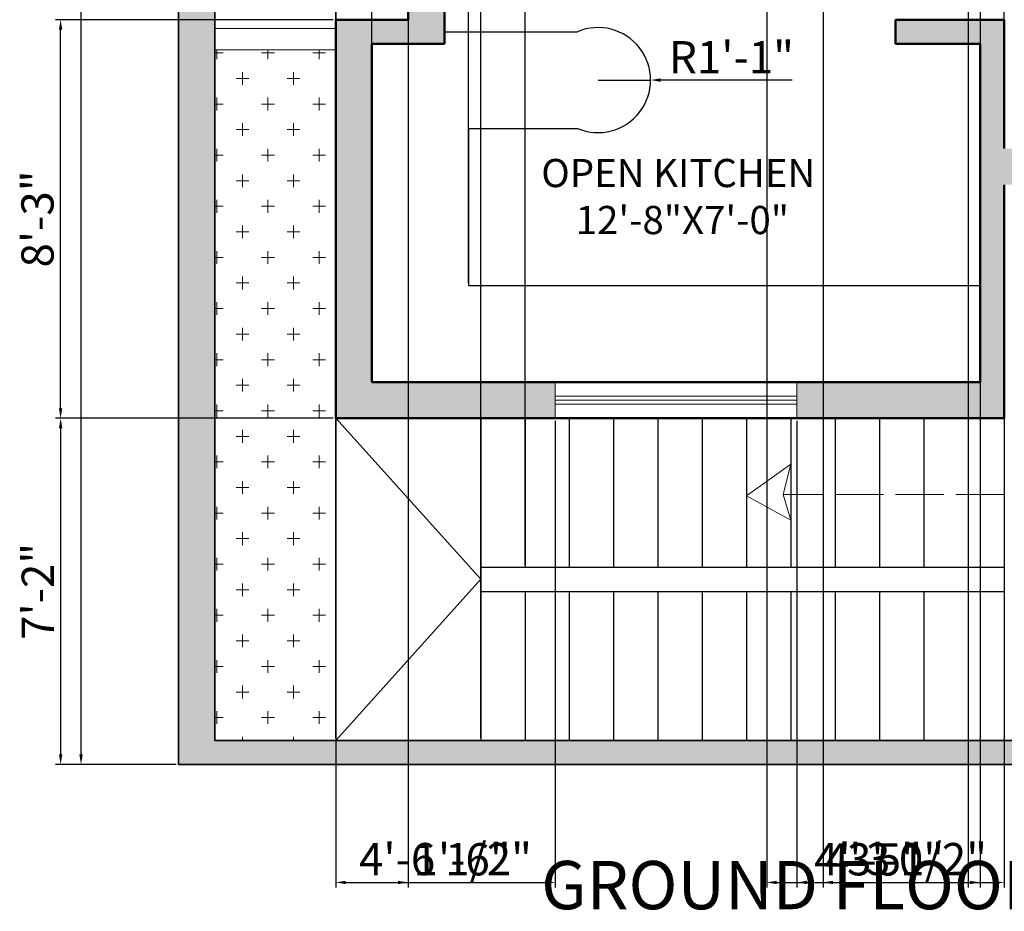
# Model space of a CAD drawing. Units: inches. Extents: x 1369 to 1844, y 2136 to 2743.
# Tile 1 of 4: x 1375 to 1620, y 2136 to 2358. Entities that reach past the tile are written whole.
import ezdxf

# ---------------------------------------------------------------- set-up
doc = ezdxf.new("R2010")
doc.units = ezdxf.units.IN
doc.linetypes.add('ACAD_ISO02W100', pattern=[15, 12, -3])
for name, color, linetype, lineweight in [('A-ANNO-DIMS', 2, 'Continuous', 18), ('A-ANNO-SYMB', 7, 'Continuous', 18), ('A-ANNO-TEXT', 7, 'Continuous', 25), ('A-AREA-IDEN', 7, 'Continuous', 25), ('A-FLOR-CASE', 8, 'Continuous', 25), ('A-FLOR-PATT', 9, 'Continuous', 13), ('A-FLOR-STRS', 7, 'Continuous', 25), ('A-FLOR-STRS-PATH', 7, 'ACAD_ISO02W100', 18), ('A-WALL', 7, 'Continuous', 50), ('C-PROP', 7, 'Continuous', 35), ('L-PLNT', 3, 'Continuous', 18)]:
    doc.layers.add(name, color=color, linetype=linetype, lineweight=lineweight)
for name, color, linetype, lineweight, true_color in [('A-GLAZ', 244, 'Continuous', 20, 0x991b1e), ('A-WALL-PATT', 251, 'Continuous', 13, 0x636466), ('C-PROP-PATT', 251, 'Continuous', 13, 0x636466), ('L-PLNT-PATT', 116, 'Continuous', 13, 0x136734)]:
    doc.layers.add(name, color=color, linetype=linetype, lineweight=lineweight, true_color=true_color)
doc.styles.get("Standard").update_dxf_attribs({"font": 'arial.ttf'})
doc.dimstyles.new('ISO-25', dxfattribs={"dimtxt": 8, "dimasz": 2.5, "dimexe": 1.25, "dimexo": 0.625, "dimtad": 1, "dimlunit": 3, "dimtxsty": 'Standard', "dimcen": 2.5, "dimadec": 0, "dimazin": 0, "dimtfac": 1, "dimtmove": 0, "dimatfit": 3, "dimfxl": 1, "dimarcsym": 0})

# ---------------------------------------------------------------- blocks, each defined once
blk = doc.blocks.new('*D12')
at = {"layer": 'A-ANNO-DIMS', "color": 0, "lineweight": -2, "transparency": 16777216}
for p, q in [((1413.89, 2682.76), (1389.03, 2682.76)), ((1390.28, 2175.26), (1390.28, 2680.26)), ((1413.89, 2172.76), (1389.03, 2172.76))]:
    blk.add_line(p, q, dxfattribs=at)
at = {"layer": 'A-ANNO-DIMS', "color": 0, "transparency": 16777216}
for points in [[(1389.86, 2680.26), (1390.69, 2680.26), (1390.28, 2682.76)], [(1389.86, 2175.26), (1390.69, 2175.26), (1390.28, 2172.76)]]:
    blk.add_solid(points, dxfattribs=at)
at = {"layer": 'Defpoints', "color": 0, "transparency": 16777216}
for p in [(1390.28, 2682.76), (1414.51, 2682.76), (1414.51, 2172.76)]:
    blk.add_point(p, dxfattribs=at)
at = {"layer": 'A-ANNO-DIMS', "color": 0, "transparency": 16777216, "insert": (1385.57, 2427.76), "char_height": 8, "attachment_point": 5, "rotation": 90}
blk.add_mtext('42\'-6"', dxfattribs=at)
blk = doc.blocks.new('WIN-60IN')
for p, q in [((3.5, 0), (3.5, 60)), ((4.5, 0), (4.5, 60)), ((5.5, 0), (5.5, 60))]:
    blk.add_line(p, q)
blk.add_lwpolyline([(0, 60), (9, 60), (9, 0), (0, 0)], close=True)
blk = doc.blocks.new('*D36')
at = {"layer": 'A-ANNO-DIMS', "color": 0, "lineweight": -2, "transparency": 16777216}
for p, q in [((1452.89, 2258.76), (1383.96, 2258.76)), ((1385.21, 2256.26), (1385.21, 2175.26)), ((1413.89, 2172.76), (1383.96, 2172.76))]:
    blk.add_line(p, q, dxfattribs=at)
at = {"layer": 'A-ANNO-DIMS', "color": 0, "transparency": 16777216}
for points in [[(1384.79, 2256.26), (1385.63, 2256.26), (1385.21, 2258.76)], [(1384.79, 2175.26), (1385.63, 2175.26), (1385.21, 2172.76)]]:
    blk.add_solid(points, dxfattribs=at)
at = {"layer": 'Defpoints', "color": 0, "transparency": 16777216}
for p in [(1453.51, 2258.76), (1385.21, 2172.76), (1414.51, 2172.76)]:
    blk.add_point(p, dxfattribs=at)
at = {"layer": 'A-ANNO-DIMS', "color": 0, "transparency": 16777216, "insert": (1380.57, 2215.76), "char_height": 8, "attachment_point": 5, "rotation": 90}
blk.add_mtext('7\'-2"', dxfattribs=at)
blk = doc.blocks.new('*D37')
at = {"layer": 'A-ANNO-DIMS', "color": 0, "lineweight": -2, "transparency": 16777216}
for p, q in [((1452.89, 2357.76), (1383.96, 2357.76)), ((1385.21, 2261.26), (1385.21, 2355.26)), ((1452.89, 2258.76), (1383.96, 2258.76))]:
    blk.add_line(p, q, dxfattribs=at)
at = {"layer": 'A-ANNO-DIMS', "color": 0, "transparency": 16777216}
for points in [[(1384.79, 2355.26), (1385.63, 2355.26), (1385.21, 2357.76)], [(1384.79, 2261.26), (1385.63, 2261.26), (1385.21, 2258.76)]]:
    blk.add_solid(points, dxfattribs=at)
at = {"layer": 'Defpoints', "color": 0, "transparency": 16777216}
for p in [(1385.21, 2357.76), (1453.51, 2357.76), (1453.51, 2258.76)]:
    blk.add_point(p, dxfattribs=at)
at = {"layer": 'A-ANNO-DIMS', "color": 0, "transparency": 16777216, "insert": (1380.5, 2308.26), "char_height": 8, "attachment_point": 5, "rotation": 90}
blk.add_mtext('8\'-3"', dxfattribs=at)
blk = doc.blocks.new('*D42')
at = {"layer": 'A-ANNO-DIMS', "color": 0, "lineweight": -2, "transparency": 16777216}
for p, q in [((1453.51, 2453.13), (1453.51, 2142.21)), ((1471.51, 2453.13), (1471.51, 2142.21)), ((1456.01, 2143.46), (1469.01, 2143.46)), ((1471.51, 2143.46), (1495.77, 2143.46))]:
    blk.add_line(p, q, dxfattribs=at)
at = {"layer": 'A-ANNO-DIMS', "color": 0, "transparency": 16777216}
for points in [[(1456.01, 2143.87), (1456.01, 2143.04), (1453.51, 2143.46)], [(1469.01, 2143.87), (1469.01, 2143.04), (1471.51, 2143.46)]]:
    blk.add_solid(points, dxfattribs=at)
at = {"layer": 'Defpoints', "color": 0, "transparency": 16777216}
for p in [(1453.51, 2453.76), (1471.51, 2453.76), (1471.51, 2143.46)]:
    blk.add_point(p, dxfattribs=at)
at = {"layer": 'A-ANNO-DIMS', "color": 0, "transparency": 16777216, "insert": (1484.89, 2148.17), "char_height": 8, "attachment_point": 5}
blk.add_mtext('1\'-6"', dxfattribs=at)
blk = doc.blocks.new('*D43')
at = {"layer": 'A-ANNO-DIMS', "color": 0, "lineweight": -2, "transparency": 16777216}
for p, q in [((1453.51, 2258.13), (1453.51, 2142.21)), ((1508.01, 2258.13), (1508.01, 2142.21)), ((1456.01, 2143.46), (1505.51, 2143.46))]:
    blk.add_line(p, q, dxfattribs=at)
at = {"layer": 'A-ANNO-DIMS', "color": 0, "transparency": 16777216}
for points in [[(1456.01, 2143.87), (1456.01, 2143.04), (1453.51, 2143.46)], [(1505.51, 2143.87), (1505.51, 2143.04), (1508.01, 2143.46)]]:
    blk.add_solid(points, dxfattribs=at)
at = {"layer": 'Defpoints', "color": 0, "transparency": 16777216}
for p in [(1453.51, 2258.76), (1508.01, 2258.76), (1508.01, 2143.46)]:
    blk.add_point(p, dxfattribs=at)
at = {"layer": 'A-ANNO-DIMS', "color": 0, "transparency": 16777216, "insert": (1480.76, 2148.22), "char_height": 8, "attachment_point": 5}
blk.add_mtext('4\'-6 1/2"', dxfattribs=at)
blk = doc.blocks.new('*D44')
at = {"layer": 'A-ANNO-DIMS', "color": 0, "lineweight": -2, "transparency": 16777216}
for p, q in [((1568.01, 2258.13), (1568.01, 2142.21)), ((1619.51, 2258.13), (1619.51, 2142.21)), ((1570.51, 2143.46), (1617.01, 2143.46))]:
    blk.add_line(p, q, dxfattribs=at)
at = {"layer": 'A-ANNO-DIMS', "color": 0, "transparency": 16777216}
for points in [[(1570.51, 2143.87), (1570.51, 2143.04), (1568.01, 2143.46)], [(1617.01, 2143.87), (1617.01, 2143.04), (1619.51, 2143.46)]]:
    blk.add_solid(points, dxfattribs=at)
at = {"layer": 'Defpoints', "color": 0, "transparency": 16777216}
for p in [(1568.01, 2258.76), (1619.51, 2258.76), (1619.51, 2143.46)]:
    blk.add_point(p, dxfattribs=at)
at = {"layer": 'A-ANNO-DIMS', "color": 0, "transparency": 16777216, "insert": (1593.76, 2148.22), "char_height": 8, "attachment_point": 5}
blk.add_mtext('4\'-3 1/2"', dxfattribs=at)
blk = doc.blocks.new('*D45')
at = {"layer": 'A-ANNO-DIMS', "color": 0, "lineweight": -2, "transparency": 16777216}
for p, q in [((1619.51, 2326.38), (1619.51, 2734.31)), ((1636.5, 2326.38), (1636.5, 2734.31)), ((1622.01, 2733.06), (1634, 2733.06)), ((1636.5, 2733.06), (1660.77, 2733.06))]:
    blk.add_line(p, q, dxfattribs=at)
at = {"layer": 'A-ANNO-DIMS', "color": 0, "transparency": 16777216}
for points in [[(1622.01, 2733.47), (1622.01, 2732.64), (1619.51, 2733.06)], [(1634, 2733.47), (1634, 2732.64), (1636.5, 2733.06)]]:
    blk.add_solid(points, dxfattribs=at)
at = {"layer": 'Defpoints', "color": 0, "transparency": 16777216}
for p in [(1636.5, 2733.06), (1619.51, 2325.76), (1636.5, 2325.76)]:
    blk.add_point(p, dxfattribs=at)
at = {"layer": 'A-ANNO-DIMS', "color": 0, "transparency": 16777216, "insert": (1649.88, 2737.77), "char_height": 8, "attachment_point": 5}
blk.add_mtext('1\'-5"', dxfattribs=at)
blk = doc.blocks.new('*D49')
at = {"layer": 'A-ANNO-DIMS', "color": 0, "lineweight": -2, "transparency": 16777216}
for p, q in [((1574.51, 2507.13), (1574.51, 2142.21)), ((1610.51, 2507.13), (1610.51, 2142.21)), ((1577.01, 2143.46), (1608.01, 2143.46))]:
    blk.add_line(p, q, dxfattribs=at)
at = {"layer": 'A-ANNO-DIMS', "color": 0, "transparency": 16777216}
for points in [[(1577.01, 2143.87), (1577.01, 2143.04), (1574.51, 2143.46)], [(1608.01, 2143.87), (1608.01, 2143.04), (1610.51, 2143.46)]]:
    blk.add_solid(points, dxfattribs=at)
at = {"layer": 'Defpoints', "color": 0, "transparency": 16777216}
for p in [(1574.51, 2507.76), (1610.51, 2507.76), (1610.51, 2143.46)]:
    blk.add_point(p, dxfattribs=at)
at = {"layer": 'A-ANNO-DIMS', "color": 0, "transparency": 16777216, "insert": (1592.51, 2148.17), "char_height": 8, "attachment_point": 5}
blk.add_mtext('3\'-0"', dxfattribs=at)
blk = doc.blocks.new('*D53')
at = {"layer": 'A-ANNO-DIMS', "color": 0, "lineweight": -2, "transparency": 16777216}
for p, q in [((1613.51, 2469.13), (1613.51, 2142.21)), ((1560.51, 2453.13), (1560.51, 2142.21)), ((1563.01, 2143.46), (1611.01, 2143.46))]:
    blk.add_line(p, q, dxfattribs=at)
at = {"layer": 'A-ANNO-DIMS', "color": 0, "transparency": 16777216}
for points in [[(1563.01, 2143.87), (1563.01, 2143.04), (1560.51, 2143.46)], [(1611.01, 2143.87), (1611.01, 2143.04), (1613.51, 2143.46)]]:
    blk.add_solid(points, dxfattribs=at)
at = {"layer": 'Defpoints', "color": 0, "transparency": 16777216}
for p in [(1613.51, 2469.76), (1560.51, 2453.76), (1613.51, 2143.46)]:
    blk.add_point(p, dxfattribs=at)
at = {"layer": 'A-ANNO-DIMS', "color": 0, "transparency": 16777216, "insert": (1587.01, 2148.15), "char_height": 8, "attachment_point": 5}
blk.add_mtext('4\'-5"', dxfattribs=at)
blk = doc.blocks.new('*D54')
at = {"layer": 'A-ANNO-DIMS', "color": 0, "lineweight": -2, "transparency": 16777216}
for p, q in [((1462.51, 2268.38), (1462.51, 2734.31)), ((1486.51, 2292.38), (1486.51, 2734.31)), ((1465.01, 2733.06), (1484.01, 2733.06))]:
    blk.add_line(p, q, dxfattribs=at)
at = {"layer": 'A-ANNO-DIMS', "color": 0, "transparency": 16777216}
for points in [[(1465.01, 2733.47), (1465.01, 2732.64), (1462.51, 2733.06)], [(1484.01, 2733.47), (1484.01, 2732.64), (1486.51, 2733.06)]]:
    blk.add_solid(points, dxfattribs=at)
at = {"layer": 'Defpoints', "color": 0, "transparency": 16777216}
for p in [(1486.51, 2733.06), (1486.51, 2291.76), (1462.51, 2267.76)]:
    blk.add_point(p, dxfattribs=at)
at = {"layer": 'A-ANNO-DIMS', "color": 0, "transparency": 16777216, "insert": (1474.51, 2737.77), "char_height": 8, "attachment_point": 5}
blk.add_mtext('2\'-0"', dxfattribs=at)
blk = doc.blocks.new('*D55')
at = {"layer": 'A-ANNO-DIMS', "color": 0, "lineweight": -2, "transparency": 16777216}
for p, q in [((1453.51, 2179.38), (1453.51, 2734.31)), ((1489.51, 2179.38), (1489.51, 2734.31)), ((1456.01, 2733.06), (1487.01, 2733.06))]:
    blk.add_line(p, q, dxfattribs=at)
at = {"layer": 'A-ANNO-DIMS', "color": 0, "transparency": 16777216}
for points in [[(1456.01, 2733.47), (1456.01, 2732.64), (1453.51, 2733.06)], [(1487.01, 2733.47), (1487.01, 2732.64), (1489.51, 2733.06)]]:
    blk.add_solid(points, dxfattribs=at)
at = {"layer": 'Defpoints', "color": 0, "transparency": 16777216}
for p in [(1489.51, 2733.06), (1453.51, 2178.76), (1489.51, 2178.76)]:
    blk.add_point(p, dxfattribs=at)
at = {"layer": 'A-ANNO-DIMS', "color": 0, "transparency": 16777216, "insert": (1471.51, 2737.77), "char_height": 8, "attachment_point": 5}
blk.add_mtext('3\'-0"', dxfattribs=at)
blk = doc.blocks.new('*D56')
at = {"layer": 'A-ANNO-DIMS', "color": 0, "lineweight": -2, "transparency": 16777216}
for p, q in [((1489.51, 2222.38), (1489.51, 2734.31)), ((1500.51, 2222.38), (1500.51, 2734.31)), ((1492.01, 2733.06), (1498.01, 2733.06)), ((1500.51, 2733.06), (1531.74, 2733.06))]:
    blk.add_line(p, q, dxfattribs=at)
at = {"layer": 'A-ANNO-DIMS', "color": 0, "transparency": 16777216}
for points in [[(1492.01, 2733.47), (1492.01, 2732.64), (1489.51, 2733.06)], [(1498.01, 2733.47), (1498.01, 2732.64), (1500.51, 2733.06)]]:
    blk.add_solid(points, dxfattribs=at)
at = {"layer": 'Defpoints', "color": 0, "transparency": 16777216}
for p in [(1500.51, 2733.06), (1489.51, 2221.76), (1500.51, 2221.76)]:
    blk.add_point(p, dxfattribs=at)
at = {"layer": 'A-ANNO-DIMS', "color": 0, "transparency": 16777216, "insert": (1517.38, 2737.77), "char_height": 8, "attachment_point": 5}
blk.add_mtext('0\'-11"', dxfattribs=at)
blk = doc.blocks.new('*D57')
at = {"layer": 'A-ANNO-DIMS', "color": 0, "lineweight": -2, "transparency": 16777216}
for p, q in [((1518.64, 2342.76), (1531.68, 2342.76)), ((1566.86, 2342.76), (1534.18, 2342.76))]:
    blk.add_line(p, q, dxfattribs=at)
at = {"layer": 'A-ANNO-DIMS', "color": 0, "transparency": 16777216}
blk.add_solid([(1534.18, 2343.17), (1534.18, 2342.34), (1531.68, 2342.76)], dxfattribs=at)
at = {"layer": 'Defpoints', "color": 0, "transparency": 16777216}
for p in [(1518.64, 2342.76), (1531.68, 2342.76)]:
    blk.add_point(p, dxfattribs=at)
at = {"layer": 'A-ANNO-DIMS', "color": 0, "transparency": 16777216, "insert": (1551.77, 2347.4), "char_height": 8, "attachment_point": 5, "rotation": 359.9999}
blk.add_mtext('R1\'-1"', dxfattribs=at)

msp = doc.modelspace()

# ---------------------------------------------------------------- hatches: boundary and pattern name
at = {"layer": 'A-WALL-PATT'}
h = msp.add_hatch(color=256, dxfattribs=at)
h.dxf.hatch_style = 1
h.paths.add_polyline_path([(1619.511, 2460.756), (1768.511, 2460.756), (1768.511, 2444.065), (1777.511, 2444.065), (1777.511, 2498.256), (1768.511, 2498.256), (1768.511, 2466.756), (1619.511, 2466.756), (1619.511, 2469.756), (1614.511, 2469.756), (1613.511, 2469.756), (1613.511, 2433.756), (1619.511, 2433.756)])
h.paths.add_polyline_path([(1480.511, 2453.756), (1560.511, 2453.756), (1560.511, 2474.756), (1556.011, 2474.756), (1554.511, 2474.756), (1554.511, 2459.756), (1462.511, 2459.756), (1462.511, 2473.256), (1453.511, 2473.256), (1453.511, 2453.756), (1471.511, 2453.756), (1471.511, 2390.756), (1480.511, 2390.756)])
h.paths.add_polyline_path([(1574.511, 2513.156), (1574.511, 2513.756), (1462.511, 2513.756), (1462.511, 2551.882), (1453.511, 2551.882), (1453.511, 2494.256), (1462.511, 2494.256), (1462.511, 2507.756), (1554.511, 2507.756), (1554.511, 2504.756), (1556.011, 2504.756), (1560.511, 2504.756), (1560.511, 2507.756), (1574.511, 2507.756)])
h.paths.add_polyline_path([(1462.511, 2351.756), (1480.511, 2351.756), (1480.511, 2357.756), (1480.511, 2360.756), (1476.011, 2360.756), (1471.511, 2360.756), (1471.511, 2357.756), (1453.511, 2357.756), (1453.511, 2258.756), (1508.011, 2258.756), (1508.011, 2267.756), (1462.511, 2267.756)])
h.paths.add_polyline_path([(1619.511, 2357.756), (1592.511, 2357.756), (1592.511, 2351.756), (1613.511, 2351.756), (1613.511, 2267.756), (1568.011, 2267.756), (1568.011, 2258.756), (1619.511, 2258.756), (1619.511, 2316.756), (1636.503, 2316.756), (1636.503, 2325.756), (1619.511, 2325.756)])
h.paths.add_polyline_path([(1717.511, 2323.956), (1717.511, 2325.756), (1696.503, 2325.756), (1696.503, 2316.756), (1717.511, 2316.756)])
h.paths.add_polyline_path([(1777.511, 2384.065), (1768.511, 2384.065), (1768.511, 2325.756), (1765.511, 2325.756), (1765.511, 2323.956), (1765.511, 2316.756), (1777.511, 2316.756)])
h.paths.add_polyline_path([(1777.511, 2652.756), (1731.511, 2652.756), (1731.511, 2643.756), (1768.511, 2643.756), (1768.511, 2595.756), (1673.511, 2595.756), (1673.511, 2598.756), (1672.011, 2598.756), (1667.511, 2598.756), (1667.511, 2595.756), (1613.511, 2595.756), (1613.511, 2513.756), (1610.511, 2513.756), (1610.511, 2513.156), (1610.511, 2507.756), (1613.511, 2507.756), (1613.511, 2505.756), (1619.511, 2505.756), (1619.511, 2589.756), (1768.511, 2589.756), (1768.511, 2558.256), (1777.511, 2558.256)])
h.paths.add_polyline_path([(1710.511, 2652.756), (1616.643, 2652.756), (1616.643, 2643.756), (1667.511, 2643.756), (1667.511, 2628.756), (1672.011, 2628.756), (1673.511, 2628.756), (1673.511, 2643.756), (1710.511, 2643.756)], flags=17)
h.paths.add_polyline_path([(1556.643, 2652.756), (1453.511, 2652.756), (1453.511, 2611.882), (1462.511, 2611.882), (1462.511, 2643.756), (1556.643, 2643.756)])
at = {"layer": 'C-PROP-PATT'}
h = msp.add_hatch(color=256, dxfattribs=at)
h.dxf.hatch_style = 1
h.paths.add_polyline_path([(1423.511, 2676.756), (1801.511, 2676.756), (1801.511, 2178.756), (1777.511, 2178.756), (1777.511, 2172.756), (1807.511, 2172.756), (1807.511, 2682.756), (1414.511, 2682.756), (1414.511, 2172.756), (1642.884, 2172.756), (1642.884, 2178.756), (1423.511, 2178.756)])
at = {"layer": 'L-PLNT-PATT'}
h = msp.add_hatch(dxfattribs=at)
h.set_pattern_fill('CROSS', color=256)
h.paths.add_polyline_path([(1453.511, 2652.756), (1777.511, 2652.756), (1788.511, 2652.756), (1788.511, 2178.756), (1801.511, 2178.756), (1801.511, 2676.756), (1423.511, 2676.756), (1423.511, 2453.756), (1453.511, 2453.756)])
h.paths.add_polyline_path([(1453.511, 2350.279), (1423.511, 2350.279), (1423.511, 2178.756), (1453.511, 2178.756), (1453.511, 2258.756)], flags=17)

# ---------------------------------------------------------------- linework, layer by layer
at = {"layer": 'A-ANNO-SYMB'}
for p, q in [((1566.511, 2247.329), (1555.511, 2239.469)), ((1564.638, 2239.82), (1566.511, 2247.329)), ((1555.511, 2239.469), (1566.511, 2233.476)), ((1566.511, 2233.476), (1564.638, 2239.82))]:
    msp.add_line(p, q, dxfattribs=at)
at = {"layer": 'A-FLOR-CASE'}
for p, q in [((1480.511, 2354.756), (1513.511, 2354.756)), ((1486.511, 2330.756), (1486.511, 2291.756)), ((1486.511, 2330.756), (1513.511, 2330.756)), ((1486.511, 2291.756), (1613.511, 2291.756))]:
    msp.add_line(p, q, dxfattribs=at)
msp.add_arc((1518.635, 2342.756), 13.048, 246.8774, 113.1226, dxfattribs=at)
at = {"layer": 'A-FLOR-PATT'}
msp.add_line((1453.511, 2355.542), (1423.511, 2355.542), dxfattribs=at)
at = {"layer": 'A-FLOR-STRS'}
for p, q in [((1619.511, 2316.756), (1619.511, 2178.756)), ((1453.511, 2258.756), (1453.511, 2178.756)), ((1489.511, 2218.756), (1453.511, 2258.756)), ((1489.511, 2258.756), (1489.511, 2178.756)), ((1500.511, 2258.756), (1500.511, 2221.756)), ((1511.511, 2258.756), (1511.511, 2221.756)), ((1522.511, 2258.756), (1522.511, 2221.756)), ((1533.511, 2258.756), (1533.511, 2221.756)), ((1544.511, 2258.756), (1544.511, 2221.756)), ((1555.511, 2258.756), (1555.511, 2221.756)), ((1566.511, 2258.756), (1566.511, 2221.756)), ((1577.511, 2258.756), (1577.511, 2221.756)), ((1588.511, 2258.756), (1588.511, 2221.756)), ((1599.511, 2258.756), (1599.511, 2221.756)), ((1610.511, 2258.756), (1610.511, 2221.756)), ((1489.511, 2221.756), (1619.511, 2221.756)), ((1489.511, 2218.756), (1453.511, 2178.756)), ((1489.511, 2215.756), (1619.511, 2215.756)), ((1500.511, 2215.756), (1500.511, 2178.756)), ((1511.511, 2215.756), (1511.511, 2178.756)), ((1522.511, 2215.756), (1522.511, 2178.756)), ((1533.511, 2215.756), (1533.511, 2178.756)), ((1544.511, 2215.756), (1544.511, 2178.756)), ((1555.511, 2215.756), (1555.511, 2178.756)), ((1566.511, 2215.756), (1566.511, 2178.756)), ((1577.511, 2215.756), (1577.511, 2178.756)), ((1588.511, 2215.756), (1588.511, 2178.756)), ((1599.511, 2215.756), (1599.511, 2178.756)), ((1610.511, 2215.756), (1610.511, 2178.756))]:
    msp.add_line(p, q, dxfattribs=at)
at = {"layer": 'A-FLOR-STRS-PATH'}
msp.add_line((1619.511, 2239.82), (1564.638, 2239.82), dxfattribs=at)
at = {"layer": 'A-WALL'}
for p, q in [((1480.511, 2453.756), (1480.511, 2357.756)), ((1471.511, 2360.756), (1471.511, 2357.756)), ((1453.511, 2357.756), (1471.511, 2357.756)), ((1453.511, 2357.756), (1453.511, 2258.756)), ((1480.511, 2357.756), (1480.511, 2351.756)), ((1592.511, 2357.756), (1619.511, 2357.756)), ((1592.511, 2351.756), (1592.511, 2357.756)), ((1619.511, 2357.756), (1619.511, 2325.756)), ((1462.511, 2351.756), (1480.511, 2351.756)), ((1462.511, 2351.756), (1462.511, 2267.756)), ((1592.511, 2351.756), (1613.511, 2351.756)), ((1613.511, 2351.756), (1613.511, 2267.756)), ((1619.511, 2316.756), (1619.511, 2258.756)), ((1462.511, 2267.756), (1613.511, 2267.756)), ((1453.511, 2258.756), (1619.511, 2258.756))]:
    msp.add_line(p, q, dxfattribs=at)
at = {"layer": 'C-PROP'}
for p, q in [((1414.511, 2682.756), (1414.511, 2172.756)), ((1423.511, 2676.756), (1423.511, 2178.756)), ((1423.511, 2178.756), (1801.511, 2178.756)), ((1414.511, 2172.756), (1807.511, 2172.756))]:
    msp.add_line(p, q, dxfattribs=at)
at = {"layer": 'L-PLNT'}
msp.add_line((1423.511, 2350.279), (1453.511, 2350.279), dxfattribs=at)

# ---------------------------------------------------------------- block references
at = {"layer": 'A-GLAZ', "rotation": 269.9999999999999}
msp.add_blockref('WIN-60IN', (1508.011, 2267.756), dxfattribs=at)

# ---------------------------------------------------------------- texts
at = {"layer": 'A-ANNO-TEXT', "insert": (1504.541, 2148.798), "char_height": 12, "attachment_point": 1}
msp.add_mtext_dynamic_manual_height_columns('GROUND FLOOR PLAN', width=194.0265, gutter_width=12.5, heights=[0], dxfattribs=at)
at = {"layer": 'A-AREA-IDEN', "insert": (1504.541, 2323.166), "char_height": 7, "attachment_point": 1}
msp.add_mtext_dynamic_manual_height_columns('OPEN KITCHEN\\P    12\'-8"X7\'-0"', width=76.85979, gutter_width=12.5, heights=[0], dxfattribs=at)

# ---------------------------------------------------------------- dimensions: what is measured, and where the dimension line sits
at = {"layer": 'A-ANNO-DIMS'}
for base, p1, p2, picture, middle in [((1489.511, 2733.056), (1453.511, 2178.756), (1489.511, 2178.756), '*D55', (1471.511, 2737.768)), ((1486.511, 2733.056), (1462.511, 2267.756), (1486.511, 2291.756), '*D54', (1474.511, 2737.766)), ((1500.511, 2733.056), (1489.511, 2221.756), (1500.511, 2221.756), '*D56', (1517.377, 2737.766)), ((1636.503, 2733.056), (1619.511, 2325.756), (1636.503, 2325.756), '*D45', (1649.884, 2737.766)), ((1610.511, 2143.456), (1574.511, 2507.756), (1610.511, 2507.756), '*D49', (1592.511, 2148.168)), ((1613.511, 2143.456), (1560.511, 2453.756), (1613.511, 2469.756), '*D53', (1587.011, 2148.149)), ((1471.511, 2143.456), (1453.511, 2453.756), (1471.511, 2453.756), '*D42', (1484.893, 2148.166)), ((1508.011, 2143.456), (1453.511, 2258.756), (1508.011, 2258.756), '*D43', (1480.761, 2148.217)), ((1619.511, 2143.456), (1568.011, 2258.756), (1619.511, 2258.756), '*D44', (1593.761, 2148.22))]:
    dim = msp.add_linear_dim(base=base, p1=p1, p2=p2, dimstyle='ISO-25', override={"dimdec": 1, "dimlfac": 1, "dimrnd": 0, "dimzin": 1, "dimdsep": 46, "dimlunit": 4, "dimfrac": 2}, dxfattribs=at)
    dim.commit()
    dim.dimension.update_dxf_attribs({"geometry": picture, "text_midpoint": middle})
for base, p1, p2, override, picture, middle in [((1390.277, 2682.756), (1414.511, 2172.756), (1414.511, 2682.756), {"dimclrd": 0, "dimclre": 0, "dimclrt": 0}, '*D12', (1385.567, 2427.756)), ((1385.211, 2357.756), (1453.511, 2258.756), (1453.511, 2357.756), {"dimdec": 1, "dimlfac": 1, "dimrnd": 0, "dimzin": 1, "dimdsep": 46, "dimlunit": 4, "dimfrac": 2}, '*D37', (1380.499, 2308.256)), ((1385.211, 2172.756), (1453.511, 2258.756), (1414.511, 2172.756), {"dimdec": 1, "dimlfac": 1, "dimrnd": 0, "dimzin": 1, "dimdsep": 46, "dimlunit": 4, "dimfrac": 2}, '*D36', (1380.57, 2215.756))]:
    dim = msp.add_linear_dim(base=base, p1=p1, p2=p2, angle=90, dimstyle='ISO-25', override=override, dxfattribs=at)
    dim.commit()
    dim.dimension.update_dxf_attribs({"geometry": picture, "text_midpoint": middle})
dim = msp.add_radius_dim(center=(1518.635, 2342.756), mpoint=(1531.683, 2342.756), dimstyle='ISO-25', override={"dimdec": 1, "dimlfac": 1, "dimrnd": 0, "dimzin": 1, "dimdsep": 46, "dimlunit": 4, "dimfrac": 2}, dxfattribs=at)
dim.commit()
dim.dimension.update_dxf_attribs({"geometry": '*D57', "text_midpoint": (1551.77, 2347.397)})

doc.saveas('drawing.dxf')
